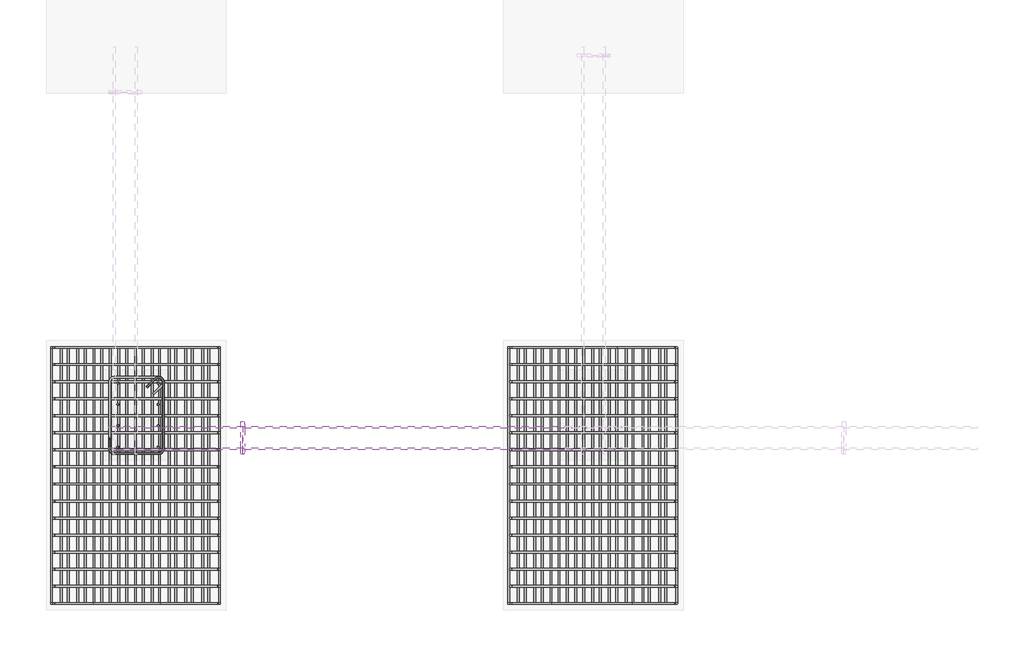
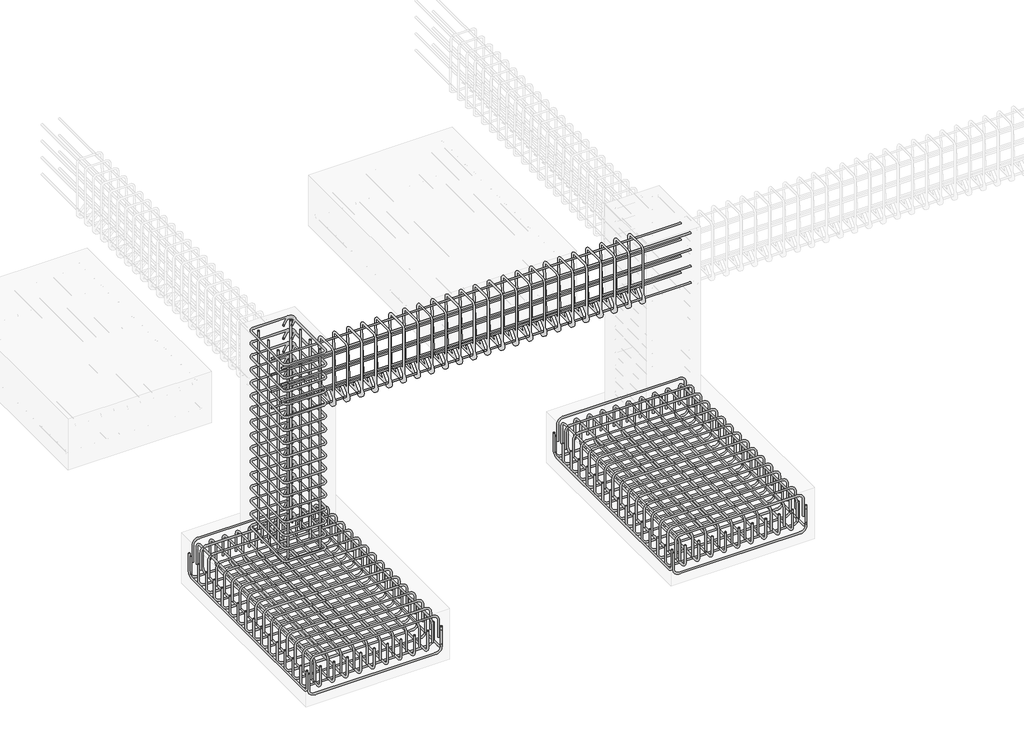
# One storey, part 2 of 16: 14 reinforcing bars.
"""IFC4 building model written with IfcOpenShell, lengths in millimetres."""

from ifc_helpers import new_model, si_unit, point, frame, origin, place, context, project, spatial, polyline, circle_curve, trimmed, segment, composite_curve, source, transform, mapped, element, save
from ifc_brep_helpers import swept_disk

model = new_model("IFC4")

# Units and contexts
model_context = context("Model", 3, world=origin())
ifc_project = project(units=[si_unit("LENGTHUNIT", "METRE", prefix="MILLI")], contexts=[model_context])

# Site, building, storey
site = spatial("IfcSite", under=ifc_project)
building = spatial("IfcBuilding", under=site)
storey = spatial("IfcBuildingStorey", under=building, Elevation=-1828.8)

# Reinforcing bars
placement = place(None, origin())
reinforcing_bar_shape = source(origin(), model_context, "Body", "SolidModel", [
    swept_disk(composite_curve([segment(polyline([(-4822.4802026, -711.9348046, -2028.4710597), (-4822.4802026, -711.9348046, -2175.7710597)]), True, "CONTINUOUS"), segment(trimmed(circle_curve(frame((-4868.8302026, -711.9348046, -2175.7710597), z_axis=(0.0, 1.0, 0.0), x_axis=(46.350000000000364, 0.0, 0.0)), 46.35), [point((-4822.4802026, -711.9348046, -2175.7710597))], [point((-4868.8302026, -711.9348046, -2222.1210597))], True, "CARTESIAN"), True, "CONTINUOUS"), segment(polyline([(-4868.8302026, -711.9348046, -2222.1210597), (-5883.4302026, -711.9348046, -2222.1210597)]), True, "CONTINUOUS"), segment(trimmed(circle_curve(frame((-5883.4302026, -711.9348046, -2175.7710597), z_axis=(0.0, 1.0, 0.0), x_axis=(0.0, 0.0, -46.34999999999991)), 46.35), [point((-5883.4302026, -711.9348046, -2222.1210597))], [point((-5929.7802026, -711.9348046, -2175.7710597))], True, "CARTESIAN"), True, "CONTINUOUS"), segment(polyline([(-5929.7802026, -711.9348046, -2175.7710597), (-5929.7802026, -711.9348046, -2028.4710597)]), True, "CONTINUOUS")], self_intersect=False), 6.35),
])
element("IfcReinforcingBar", 1, at=placement, inside=storey, context=model_context, shape_type="MappedRepresentation", body=[
    mapped(reinforcing_bar_shape, transform((0.0, 0.0, 0.0), x_axis=(1.0, 0.0, 0.0), y_axis=(0.0, 1.0, 0.0), z_axis=(0.0, 0.0, 1.0))),
    mapped(reinforcing_bar_shape, transform((0.0, -113.82, 0.0), x_axis=(1.0, 0.0, 0.0), y_axis=(0.0, 1.0, 0.0), z_axis=(0.0, 0.0, 1.0))),
    mapped(reinforcing_bar_shape, transform((0.0, -227.64, 0.0), x_axis=(1.0, 0.0, 0.0), y_axis=(0.0, 1.0, 0.0), z_axis=(0.0, 0.0, 1.0))),
    mapped(reinforcing_bar_shape, transform((0.0, -341.46, 0.0), x_axis=(1.0, 0.0, 0.0), y_axis=(0.0, 1.0, 0.0), z_axis=(0.0, 0.0, 1.0))),
    mapped(reinforcing_bar_shape, transform((0.0, -455.28, 0.0), x_axis=(1.0, 0.0, 0.0), y_axis=(0.0, 1.0, 0.0), z_axis=(0.0, 0.0, 1.0))),
    mapped(reinforcing_bar_shape, transform((0.0, -569.1, 0.0), x_axis=(1.0, 0.0, 0.0), y_axis=(0.0, 1.0, 0.0), z_axis=(0.0, 0.0, 1.0))),
    mapped(reinforcing_bar_shape, transform((0.0, -682.92, 0.0), x_axis=(1.0, 0.0, 0.0), y_axis=(0.0, 1.0, 0.0), z_axis=(0.0, 0.0, 1.0))),
    mapped(reinforcing_bar_shape, transform((0.0, -796.74, 0.0), x_axis=(1.0, 0.0, 0.0), y_axis=(0.0, 1.0, 0.0), z_axis=(0.0, 0.0, 1.0))),
    mapped(reinforcing_bar_shape, transform((0.0, -910.56, 0.0), x_axis=(1.0, 0.0, 0.0), y_axis=(0.0, 1.0, 0.0), z_axis=(0.0, 0.0, 1.0))),
    mapped(reinforcing_bar_shape, transform((0.0, -1024.38, 0.0), x_axis=(1.0, 0.0, 0.0), y_axis=(0.0, 1.0, 0.0), z_axis=(0.0, 0.0, 1.0))),
    mapped(reinforcing_bar_shape, transform((0.0, -1138.2, 0.0), x_axis=(1.0, 0.0, 0.0), y_axis=(0.0, 1.0, 0.0), z_axis=(0.0, 0.0, 1.0))),
    mapped(reinforcing_bar_shape, transform((0.0, -1252.02, 0.0), x_axis=(1.0, 0.0, 0.0), y_axis=(0.0, 1.0, 0.0), z_axis=(0.0, 0.0, 1.0))),
    mapped(reinforcing_bar_shape, transform((0.0, -1365.84, 0.0), x_axis=(1.0, 0.0, 0.0), y_axis=(0.0, 1.0, 0.0), z_axis=(0.0, 0.0, 1.0))),
    mapped(reinforcing_bar_shape, transform((0.0, -1479.66, 0.0), x_axis=(1.0, 0.0, 0.0), y_axis=(0.0, 1.0, 0.0), z_axis=(0.0, 0.0, 1.0))),
    mapped(reinforcing_bar_shape, transform((0.0, -1593.48, 0.0), x_axis=(1.0, 0.0, 0.0), y_axis=(0.0, 1.0, 0.0), z_axis=(0.0, 0.0, 1.0))),
    mapped(reinforcing_bar_shape, transform((0.0, -1707.3, 0.0), x_axis=(1.0, 0.0, 0.0), y_axis=(0.0, 1.0, 0.0), z_axis=(0.0, 0.0, 1.0))),
])
reinforcing_bar_2_shape = source(origin(), model_context, "Body", "SolidModel", [
    swept_disk(composite_curve([segment(polyline([(-5911.3242766, -711.9348046, -2081.4939987), (-5911.3242766, -711.9348046, -1934.1939987)]), True, "CONTINUOUS"), segment(trimmed(circle_curve(frame((-5864.9742766, -711.9348046, -1934.1939987), z_axis=(0.0, 1.0, 0.0), x_axis=(-46.350000000000364, 0.0, 0.0)), 46.35), [point((-5911.3242766, -711.9348046, -1934.1939987))], [point((-5864.9742766, -711.9348046, -1887.8439987))], True, "CARTESIAN"), True, "CONTINUOUS"), segment(polyline([(-5864.9742766, -711.9348046, -1887.8439987), (-4891.2549298, -711.9348046, -1887.8439987)]), True, "CONTINUOUS"), segment(trimmed(circle_curve(frame((-4891.2549298, -711.9348046, -1934.1939987), z_axis=(0.0, 1.0, 0.0), x_axis=(0.0, 0.0, 46.350000000000136)), 46.35), [point((-4891.2549298, -711.9348046, -1887.8439987))], [point((-4844.9049298, -711.9348046, -1934.1939987))], True, "CARTESIAN"), True, "CONTINUOUS"), segment(polyline([(-4844.9049298, -711.9348046, -1934.1939987), (-4844.9049298, -711.9348046, -2081.4939987)]), True, "CONTINUOUS")], self_intersect=False), 6.35),
])
element("IfcReinforcingBar", 2, at=placement, inside=storey, context=model_context, shape_type="MappedRepresentation", body=[
    mapped(reinforcing_bar_2_shape, transform((0.0, 0.0, 0.0), x_axis=(1.0, 0.0, 0.0), y_axis=(0.0, 1.0, 0.0), z_axis=(0.0, 0.0, 1.0))),
    mapped(reinforcing_bar_2_shape, transform((0.0, -113.82, 0.0), x_axis=(1.0, 0.0, 0.0), y_axis=(0.0, 1.0, 0.0), z_axis=(0.0, 0.0, 1.0))),
    mapped(reinforcing_bar_2_shape, transform((0.0, -227.64, 0.0), x_axis=(1.0, 0.0, 0.0), y_axis=(0.0, 1.0, 0.0), z_axis=(0.0, 0.0, 1.0))),
    mapped(reinforcing_bar_2_shape, transform((0.0, -341.46, 0.0), x_axis=(1.0, 0.0, 0.0), y_axis=(0.0, 1.0, 0.0), z_axis=(0.0, 0.0, 1.0))),
    mapped(reinforcing_bar_2_shape, transform((0.0, -455.28, 0.0), x_axis=(1.0, 0.0, 0.0), y_axis=(0.0, 1.0, 0.0), z_axis=(0.0, 0.0, 1.0))),
    mapped(reinforcing_bar_2_shape, transform((0.0, -569.1, 0.0), x_axis=(1.0, 0.0, 0.0), y_axis=(0.0, 1.0, 0.0), z_axis=(0.0, 0.0, 1.0))),
    mapped(reinforcing_bar_2_shape, transform((0.0, -682.92, 0.0), x_axis=(1.0, 0.0, 0.0), y_axis=(0.0, 1.0, 0.0), z_axis=(0.0, 0.0, 1.0))),
    mapped(reinforcing_bar_2_shape, transform((0.0, -796.74, 0.0), x_axis=(1.0, 0.0, 0.0), y_axis=(0.0, 1.0, 0.0), z_axis=(0.0, 0.0, 1.0))),
    mapped(reinforcing_bar_2_shape, transform((0.0, -910.56, 0.0), x_axis=(1.0, 0.0, 0.0), y_axis=(0.0, 1.0, 0.0), z_axis=(0.0, 0.0, 1.0))),
    mapped(reinforcing_bar_2_shape, transform((0.0, -1024.38, 0.0), x_axis=(1.0, 0.0, 0.0), y_axis=(0.0, 1.0, 0.0), z_axis=(0.0, 0.0, 1.0))),
    mapped(reinforcing_bar_2_shape, transform((0.0, -1138.2, 0.0), x_axis=(1.0, 0.0, 0.0), y_axis=(0.0, 1.0, 0.0), z_axis=(0.0, 0.0, 1.0))),
    mapped(reinforcing_bar_2_shape, transform((0.0, -1252.02, 0.0), x_axis=(1.0, 0.0, 0.0), y_axis=(0.0, 1.0, 0.0), z_axis=(0.0, 0.0, 1.0))),
    mapped(reinforcing_bar_2_shape, transform((0.0, -1365.84, 0.0), x_axis=(1.0, 0.0, 0.0), y_axis=(0.0, 1.0, 0.0), z_axis=(0.0, 0.0, 1.0))),
    mapped(reinforcing_bar_2_shape, transform((0.0, -1479.66, 0.0), x_axis=(1.0, 0.0, 0.0), y_axis=(0.0, 1.0, 0.0), z_axis=(0.0, 0.0, 1.0))),
    mapped(reinforcing_bar_2_shape, transform((0.0, -1593.48, 0.0), x_axis=(1.0, 0.0, 0.0), y_axis=(0.0, 1.0, 0.0), z_axis=(0.0, 0.0, 1.0))),
    mapped(reinforcing_bar_2_shape, transform((0.0, -1707.3, 0.0), x_axis=(1.0, 0.0, 0.0), y_axis=(0.0, 1.0, 0.0), z_axis=(0.0, 0.0, 1.0))),
])
reinforcing_bar_3_shape = source(origin(), model_context, "Body", "SolidModel", [
    swept_disk(composite_curve([segment(polyline([(-4894.8565936, -711.9348046, -2112.6585679), (-4894.8565936, -711.9348046, -1965.3585679)]), True, "CONTINUOUS"), segment(trimmed(circle_curve(frame((-4894.8565936, -758.2848046, -1965.3585679), z_axis=(1.0, 0.0, 0.0), x_axis=(0.0, 46.35000000000002, 0.0)), 46.35), [point((-4894.8565936, -711.9348046, -1965.3585679))], [point((-4894.8565936, -758.2848046, -1919.0085679))], True, "CARTESIAN"), True, "CONTINUOUS"), segment(polyline([(-4894.8565936, -758.2848046, -1919.0085679), (-4894.8565936, -2372.8848046, -1919.0085679)]), True, "CONTINUOUS"), segment(trimmed(circle_curve(frame((-4894.8565936, -2372.8848046, -1965.3585679), z_axis=(1.0, 0.0, 0.0), x_axis=(0.0, 0.0, 46.350000000000136)), 46.35), [point((-4894.8565936, -2372.8848046, -1919.0085679))], [point((-4894.8565936, -2419.2348046, -1965.3585679))], True, "CARTESIAN"), True, "CONTINUOUS"), segment(polyline([(-4894.8565936, -2419.2348046, -1965.3585679), (-4894.8565936, -2419.2348046, -2112.6585679)]), True, "CONTINUOUS")], self_intersect=False), 6.35),
])
element("IfcReinforcingBar", 3, at=placement, inside=storey, context=model_context, shape_type="MappedRepresentation", body=[
    mapped(reinforcing_bar_3_shape, transform((0.0, 0.0, 0.0), x_axis=(1.0, 0.0, 0.0), y_axis=(0.0, 1.0, 0.0), z_axis=(0.0, 0.0, 1.0))),
    mapped(reinforcing_bar_3_shape, transform((-109.2679104, 0.0, 0.0), x_axis=(1.0, 0.0, 0.0), y_axis=(0.0, 1.0, 0.0), z_axis=(0.0, 0.0, 1.0))),
    mapped(reinforcing_bar_3_shape, transform((-218.5358207, 0.0, 0.0), x_axis=(1.0, 0.0, 0.0), y_axis=(0.0, 1.0, 0.0), z_axis=(0.0, 0.0, 1.0))),
    mapped(reinforcing_bar_3_shape, transform((-327.8037311, 0.0, 0.0), x_axis=(1.0, 0.0, 0.0), y_axis=(0.0, 1.0, 0.0), z_axis=(0.0, 0.0, 1.0))),
    mapped(reinforcing_bar_3_shape, transform((-437.0716415, 0.0, 0.0), x_axis=(1.0, 0.0, 0.0), y_axis=(0.0, 1.0, 0.0), z_axis=(0.0, 0.0, 1.0))),
    mapped(reinforcing_bar_3_shape, transform((-546.3395518, 0.0, 0.0), x_axis=(1.0, 0.0, 0.0), y_axis=(0.0, 1.0, 0.0), z_axis=(0.0, 0.0, 1.0))),
    mapped(reinforcing_bar_3_shape, transform((-655.6074622, 0.0, 0.0), x_axis=(1.0, 0.0, 0.0), y_axis=(0.0, 1.0, 0.0), z_axis=(0.0, 0.0, 1.0))),
    mapped(reinforcing_bar_3_shape, transform((-764.8753726, 0.0, 0.0), x_axis=(1.0, 0.0, 0.0), y_axis=(0.0, 1.0, 0.0), z_axis=(0.0, 0.0, 1.0))),
    mapped(reinforcing_bar_3_shape, transform((-874.1432829, 0.0, 0.0), x_axis=(1.0, 0.0, 0.0), y_axis=(0.0, 1.0, 0.0), z_axis=(0.0, 0.0, 1.0))),
    mapped(reinforcing_bar_3_shape, transform((-983.4111933, 0.0, 0.0), x_axis=(1.0, 0.0, 0.0), y_axis=(0.0, 1.0, 0.0), z_axis=(0.0, 0.0, 1.0))),
])
reinforcing_bar_4_shape = source(origin(), model_context, "Body", "SolidModel", [
    swept_disk(composite_curve([segment(polyline([(-5943.0342668, -711.9348046, -1996.4434391), (-5943.0342668, -711.9348046, -2143.7434391)]), True, "CONTINUOUS"), segment(trimmed(circle_curve(frame((-5943.0342668, -758.2848046, -2143.7434391), z_axis=(-1.0, 0.0, 0.0), x_axis=(0.0, 46.35000000000002, 0.0)), 46.35), [point((-5943.0342668, -711.9348046, -2143.7434391))], [point((-5943.0342668, -758.2848046, -2190.0934391))], True, "CARTESIAN"), True, "CONTINUOUS"), segment(polyline([(-5943.0342668, -758.2848046, -2190.0934391), (-5943.0342668, -2372.8848046, -2190.0934391)]), True, "CONTINUOUS"), segment(trimmed(circle_curve(frame((-5943.0342668, -2372.8848046, -2143.7434391), z_axis=(-1.0, 0.0, 0.0), x_axis=(0.0, 0.0, -46.34999999999991)), 46.35), [point((-5943.0342668, -2372.8848046, -2190.0934391))], [point((-5943.0342668, -2419.2348046, -2143.7434391))], True, "CARTESIAN"), True, "CONTINUOUS"), segment(polyline([(-5943.0342668, -2419.2348046, -2143.7434391), (-5943.0342668, -2419.2348046, -1996.4434391)]), True, "CONTINUOUS")], self_intersect=False), 6.35),
])
element("IfcReinforcingBar", 4, at=placement, inside=storey, context=model_context, shape_type="MappedRepresentation", body=[
    mapped(reinforcing_bar_4_shape, transform((0.0, 0.0, 0.0), x_axis=(1.0, 0.0, 0.0), y_axis=(0.0, 1.0, 0.0), z_axis=(0.0, 0.0, 1.0))),
    mapped(reinforcing_bar_4_shape, transform((112.0554064, 0.0, 0.0), x_axis=(1.0, 0.0, 0.0), y_axis=(0.0, 1.0, 0.0), z_axis=(0.0, 0.0, 1.0))),
    mapped(reinforcing_bar_4_shape, transform((224.1108128, 0.0, 0.0), x_axis=(1.0, 0.0, 0.0), y_axis=(0.0, 1.0, 0.0), z_axis=(0.0, 0.0, 1.0))),
    mapped(reinforcing_bar_4_shape, transform((336.1662192, 0.0, 0.0), x_axis=(1.0, 0.0, 0.0), y_axis=(0.0, 1.0, 0.0), z_axis=(0.0, 0.0, 1.0))),
    mapped(reinforcing_bar_4_shape, transform((448.2216256, 0.0, 0.0), x_axis=(1.0, 0.0, 0.0), y_axis=(0.0, 1.0, 0.0), z_axis=(0.0, 0.0, 1.0))),
    mapped(reinforcing_bar_4_shape, transform((560.2770321, 0.0, 0.0), x_axis=(1.0, 0.0, 0.0), y_axis=(0.0, 1.0, 0.0), z_axis=(0.0, 0.0, 1.0))),
    mapped(reinforcing_bar_4_shape, transform((672.3324385, 0.0, 0.0), x_axis=(1.0, 0.0, 0.0), y_axis=(0.0, 1.0, 0.0), z_axis=(0.0, 0.0, 1.0))),
    mapped(reinforcing_bar_4_shape, transform((784.3878449, 0.0, 0.0), x_axis=(1.0, 0.0, 0.0), y_axis=(0.0, 1.0, 0.0), z_axis=(0.0, 0.0, 1.0))),
    mapped(reinforcing_bar_4_shape, transform((896.4432513, 0.0, 0.0), x_axis=(1.0, 0.0, 0.0), y_axis=(0.0, 1.0, 0.0), z_axis=(0.0, 0.0, 1.0))),
    mapped(reinforcing_bar_4_shape, transform((1008.4986577, 0.0, 0.0), x_axis=(1.0, 0.0, 0.0), y_axis=(0.0, 1.0, 0.0), z_axis=(0.0, 0.0, 1.0))),
    mapped(reinforcing_bar_4_shape, transform((1120.5540641, 0.0, 0.0), x_axis=(1.0, 0.0, 0.0), y_axis=(0.0, 1.0, 0.0), z_axis=(0.0, 0.0, 1.0))),
])
reinforcing_bar_5_shape = source(origin(), model_context, "Body", "SolidModel", [
    swept_disk(composite_curve([segment(polyline([(-1774.4802026, -711.9348046, -2028.4710597), (-1774.4802026, -711.9348046, -2175.7710597)]), True, "CONTINUOUS"), segment(trimmed(circle_curve(frame((-1820.8302026, -711.9348046, -2175.7710597), z_axis=(0.0, 1.0, 0.0), x_axis=(46.34999999999991, 0.0, 0.0)), 46.35), [point((-1774.4802026, -711.9348046, -2175.7710597))], [point((-1820.8302026, -711.9348046, -2222.1210597))], True, "CARTESIAN"), True, "CONTINUOUS"), segment(polyline([(-1820.8302026, -711.9348046, -2222.1210597), (-2835.4302026, -711.9348046, -2222.1210597)]), True, "CONTINUOUS"), segment(trimmed(circle_curve(frame((-2835.4302026, -711.9348046, -2175.7710597), z_axis=(0.0, 1.0, 0.0), x_axis=(0.0, 0.0, -46.34999999999991)), 46.35), [point((-2835.4302026, -711.9348046, -2222.1210597))], [point((-2881.7802026, -711.9348046, -2175.7710597))], True, "CARTESIAN"), True, "CONTINUOUS"), segment(polyline([(-2881.7802026, -711.9348046, -2175.7710597), (-2881.7802026, -711.9348046, -2028.4710597)]), True, "CONTINUOUS")], self_intersect=False), 6.35),
])
element("IfcReinforcingBar", 5, at=placement, inside=storey, context=model_context, shape_type="MappedRepresentation", body=[
    mapped(reinforcing_bar_5_shape, transform((0.0, 0.0, 0.0), x_axis=(1.0, 0.0, 0.0), y_axis=(0.0, 1.0, 0.0), z_axis=(0.0, 0.0, 1.0))),
    mapped(reinforcing_bar_5_shape, transform((0.0, -113.82, 0.0), x_axis=(1.0, 0.0, 0.0), y_axis=(0.0, 1.0, 0.0), z_axis=(0.0, 0.0, 1.0))),
    mapped(reinforcing_bar_5_shape, transform((0.0, -227.64, 0.0), x_axis=(1.0, 0.0, 0.0), y_axis=(0.0, 1.0, 0.0), z_axis=(0.0, 0.0, 1.0))),
    mapped(reinforcing_bar_5_shape, transform((0.0, -341.46, 0.0), x_axis=(1.0, 0.0, 0.0), y_axis=(0.0, 1.0, 0.0), z_axis=(0.0, 0.0, 1.0))),
    mapped(reinforcing_bar_5_shape, transform((0.0, -455.28, 0.0), x_axis=(1.0, 0.0, 0.0), y_axis=(0.0, 1.0, 0.0), z_axis=(0.0, 0.0, 1.0))),
    mapped(reinforcing_bar_5_shape, transform((0.0, -569.1, 0.0), x_axis=(1.0, 0.0, 0.0), y_axis=(0.0, 1.0, 0.0), z_axis=(0.0, 0.0, 1.0))),
    mapped(reinforcing_bar_5_shape, transform((0.0, -682.92, 0.0), x_axis=(1.0, 0.0, 0.0), y_axis=(0.0, 1.0, 0.0), z_axis=(0.0, 0.0, 1.0))),
    mapped(reinforcing_bar_5_shape, transform((0.0, -796.74, 0.0), x_axis=(1.0, 0.0, 0.0), y_axis=(0.0, 1.0, 0.0), z_axis=(0.0, 0.0, 1.0))),
    mapped(reinforcing_bar_5_shape, transform((0.0, -910.56, 0.0), x_axis=(1.0, 0.0, 0.0), y_axis=(0.0, 1.0, 0.0), z_axis=(0.0, 0.0, 1.0))),
    mapped(reinforcing_bar_5_shape, transform((0.0, -1024.38, 0.0), x_axis=(1.0, 0.0, 0.0), y_axis=(0.0, 1.0, 0.0), z_axis=(0.0, 0.0, 1.0))),
    mapped(reinforcing_bar_5_shape, transform((0.0, -1138.2, 0.0), x_axis=(1.0, 0.0, 0.0), y_axis=(0.0, 1.0, 0.0), z_axis=(0.0, 0.0, 1.0))),
    mapped(reinforcing_bar_5_shape, transform((0.0, -1252.02, 0.0), x_axis=(1.0, 0.0, 0.0), y_axis=(0.0, 1.0, 0.0), z_axis=(0.0, 0.0, 1.0))),
    mapped(reinforcing_bar_5_shape, transform((0.0, -1365.84, 0.0), x_axis=(1.0, 0.0, 0.0), y_axis=(0.0, 1.0, 0.0), z_axis=(0.0, 0.0, 1.0))),
    mapped(reinforcing_bar_5_shape, transform((0.0, -1479.66, 0.0), x_axis=(1.0, 0.0, 0.0), y_axis=(0.0, 1.0, 0.0), z_axis=(0.0, 0.0, 1.0))),
    mapped(reinforcing_bar_5_shape, transform((0.0, -1593.48, 0.0), x_axis=(1.0, 0.0, 0.0), y_axis=(0.0, 1.0, 0.0), z_axis=(0.0, 0.0, 1.0))),
    mapped(reinforcing_bar_5_shape, transform((0.0, -1707.3, 0.0), x_axis=(1.0, 0.0, 0.0), y_axis=(0.0, 1.0, 0.0), z_axis=(0.0, 0.0, 1.0))),
])
reinforcing_bar_6_shape = source(origin(), model_context, "Body", "SolidModel", [
    swept_disk(composite_curve([segment(polyline([(-2863.3242766, -711.9348046, -2081.4939987), (-2863.3242766, -711.9348046, -1934.1939987)]), True, "CONTINUOUS"), segment(trimmed(circle_curve(frame((-2816.9742766, -711.9348046, -1934.1939987), z_axis=(0.0, 1.0, 0.0), x_axis=(-46.34999999999991, 0.0, 0.0)), 46.35), [point((-2863.3242766, -711.9348046, -1934.1939987))], [point((-2816.9742766, -711.9348046, -1887.8439987))], True, "CARTESIAN"), True, "CONTINUOUS"), segment(polyline([(-2816.9742766, -711.9348046, -1887.8439987), (-1843.2549298, -711.9348046, -1887.8439987)]), True, "CONTINUOUS"), segment(trimmed(circle_curve(frame((-1843.2549298, -711.9348046, -1934.1939987), z_axis=(0.0, 1.0, 0.0), x_axis=(0.0, 0.0, 46.350000000000136)), 46.35), [point((-1843.2549298, -711.9348046, -1887.8439987))], [point((-1796.9049298, -711.9348046, -1934.1939987))], True, "CARTESIAN"), True, "CONTINUOUS"), segment(polyline([(-1796.9049298, -711.9348046, -1934.1939987), (-1796.9049298, -711.9348046, -2081.4939987)]), True, "CONTINUOUS")], self_intersect=False), 6.35),
])
element("IfcReinforcingBar", 6, at=placement, inside=storey, context=model_context, shape_type="MappedRepresentation", body=[
    mapped(reinforcing_bar_6_shape, transform((0.0, 0.0, 0.0), x_axis=(1.0, 0.0, 0.0), y_axis=(0.0, 1.0, 0.0), z_axis=(0.0, 0.0, 1.0))),
    mapped(reinforcing_bar_6_shape, transform((0.0, -113.82, 0.0), x_axis=(1.0, 0.0, 0.0), y_axis=(0.0, 1.0, 0.0), z_axis=(0.0, 0.0, 1.0))),
    mapped(reinforcing_bar_6_shape, transform((0.0, -227.64, 0.0), x_axis=(1.0, 0.0, 0.0), y_axis=(0.0, 1.0, 0.0), z_axis=(0.0, 0.0, 1.0))),
    mapped(reinforcing_bar_6_shape, transform((0.0, -341.46, 0.0), x_axis=(1.0, 0.0, 0.0), y_axis=(0.0, 1.0, 0.0), z_axis=(0.0, 0.0, 1.0))),
    mapped(reinforcing_bar_6_shape, transform((0.0, -455.28, 0.0), x_axis=(1.0, 0.0, 0.0), y_axis=(0.0, 1.0, 0.0), z_axis=(0.0, 0.0, 1.0))),
    mapped(reinforcing_bar_6_shape, transform((0.0, -569.1, 0.0), x_axis=(1.0, 0.0, 0.0), y_axis=(0.0, 1.0, 0.0), z_axis=(0.0, 0.0, 1.0))),
    mapped(reinforcing_bar_6_shape, transform((0.0, -682.92, 0.0), x_axis=(1.0, 0.0, 0.0), y_axis=(0.0, 1.0, 0.0), z_axis=(0.0, 0.0, 1.0))),
    mapped(reinforcing_bar_6_shape, transform((0.0, -796.74, 0.0), x_axis=(1.0, 0.0, 0.0), y_axis=(0.0, 1.0, 0.0), z_axis=(0.0, 0.0, 1.0))),
    mapped(reinforcing_bar_6_shape, transform((0.0, -910.56, 0.0), x_axis=(1.0, 0.0, 0.0), y_axis=(0.0, 1.0, 0.0), z_axis=(0.0, 0.0, 1.0))),
    mapped(reinforcing_bar_6_shape, transform((0.0, -1024.38, 0.0), x_axis=(1.0, 0.0, 0.0), y_axis=(0.0, 1.0, 0.0), z_axis=(0.0, 0.0, 1.0))),
    mapped(reinforcing_bar_6_shape, transform((0.0, -1138.2, 0.0), x_axis=(1.0, 0.0, 0.0), y_axis=(0.0, 1.0, 0.0), z_axis=(0.0, 0.0, 1.0))),
    mapped(reinforcing_bar_6_shape, transform((0.0, -1252.02, 0.0), x_axis=(1.0, 0.0, 0.0), y_axis=(0.0, 1.0, 0.0), z_axis=(0.0, 0.0, 1.0))),
    mapped(reinforcing_bar_6_shape, transform((0.0, -1365.84, 0.0), x_axis=(1.0, 0.0, 0.0), y_axis=(0.0, 1.0, 0.0), z_axis=(0.0, 0.0, 1.0))),
    mapped(reinforcing_bar_6_shape, transform((0.0, -1479.66, 0.0), x_axis=(1.0, 0.0, 0.0), y_axis=(0.0, 1.0, 0.0), z_axis=(0.0, 0.0, 1.0))),
    mapped(reinforcing_bar_6_shape, transform((0.0, -1593.48, 0.0), x_axis=(1.0, 0.0, 0.0), y_axis=(0.0, 1.0, 0.0), z_axis=(0.0, 0.0, 1.0))),
    mapped(reinforcing_bar_6_shape, transform((0.0, -1707.3, 0.0), x_axis=(1.0, 0.0, 0.0), y_axis=(0.0, 1.0, 0.0), z_axis=(0.0, 0.0, 1.0))),
])
reinforcing_bar_7_shape = source(origin(), model_context, "Body", "SolidModel", [
    swept_disk(composite_curve([segment(polyline([(-1846.8565936, -711.9348046, -2112.6585679), (-1846.8565936, -711.9348046, -1965.3585679)]), True, "CONTINUOUS"), segment(trimmed(circle_curve(frame((-1846.8565936, -758.2848046, -1965.3585679), z_axis=(1.0, 0.0, 0.0), x_axis=(0.0, 46.35000000000002, 0.0)), 46.35), [point((-1846.8565936, -711.9348046, -1965.3585679))], [point((-1846.8565936, -758.2848046, -1919.0085679))], True, "CARTESIAN"), True, "CONTINUOUS"), segment(polyline([(-1846.8565936, -758.2848046, -1919.0085679), (-1846.8565936, -2372.8848046, -1919.0085679)]), True, "CONTINUOUS"), segment(trimmed(circle_curve(frame((-1846.8565936, -2372.8848046, -1965.3585679), z_axis=(1.0, 0.0, 0.0), x_axis=(0.0, 0.0, 46.350000000000136)), 46.35), [point((-1846.8565936, -2372.8848046, -1919.0085679))], [point((-1846.8565936, -2419.2348046, -1965.3585679))], True, "CARTESIAN"), True, "CONTINUOUS"), segment(polyline([(-1846.8565936, -2419.2348046, -1965.3585679), (-1846.8565936, -2419.2348046, -2112.6585679)]), True, "CONTINUOUS")], self_intersect=False), 6.35),
])
element("IfcReinforcingBar", 7, at=placement, inside=storey, context=model_context, shape_type="MappedRepresentation", body=[
    mapped(reinforcing_bar_7_shape, transform((0.0, 0.0, 0.0), x_axis=(1.0, 0.0, 0.0), y_axis=(0.0, 1.0, 0.0), z_axis=(0.0, 0.0, 1.0))),
    mapped(reinforcing_bar_7_shape, transform((-109.2679104, 0.0, 0.0), x_axis=(1.0, 0.0, 0.0), y_axis=(0.0, 1.0, 0.0), z_axis=(0.0, 0.0, 1.0))),
    mapped(reinforcing_bar_7_shape, transform((-218.5358207, 0.0, 0.0), x_axis=(1.0, 0.0, 0.0), y_axis=(0.0, 1.0, 0.0), z_axis=(0.0, 0.0, 1.0))),
    mapped(reinforcing_bar_7_shape, transform((-327.8037311, 0.0, 0.0), x_axis=(1.0, 0.0, 0.0), y_axis=(0.0, 1.0, 0.0), z_axis=(0.0, 0.0, 1.0))),
    mapped(reinforcing_bar_7_shape, transform((-437.0716415, 0.0, 0.0), x_axis=(1.0, 0.0, 0.0), y_axis=(0.0, 1.0, 0.0), z_axis=(0.0, 0.0, 1.0))),
    mapped(reinforcing_bar_7_shape, transform((-546.3395518, 0.0, 0.0), x_axis=(1.0, 0.0, 0.0), y_axis=(0.0, 1.0, 0.0), z_axis=(0.0, 0.0, 1.0))),
    mapped(reinforcing_bar_7_shape, transform((-655.6074622, 0.0, 0.0), x_axis=(1.0, 0.0, 0.0), y_axis=(0.0, 1.0, 0.0), z_axis=(0.0, 0.0, 1.0))),
    mapped(reinforcing_bar_7_shape, transform((-764.8753726, 0.0, 0.0), x_axis=(1.0, 0.0, 0.0), y_axis=(0.0, 1.0, 0.0), z_axis=(0.0, 0.0, 1.0))),
    mapped(reinforcing_bar_7_shape, transform((-874.1432829, 0.0, 0.0), x_axis=(1.0, 0.0, 0.0), y_axis=(0.0, 1.0, 0.0), z_axis=(0.0, 0.0, 1.0))),
    mapped(reinforcing_bar_7_shape, transform((-983.4111933, 0.0, 0.0), x_axis=(1.0, 0.0, 0.0), y_axis=(0.0, 1.0, 0.0), z_axis=(0.0, 0.0, 1.0))),
])
reinforcing_bar_8_shape = source(origin(), model_context, "Body", "SolidModel", [
    swept_disk(composite_curve([segment(polyline([(-2895.0342668, -711.9348046, -1996.4434391), (-2895.0342668, -711.9348046, -2143.7434391)]), True, "CONTINUOUS"), segment(trimmed(circle_curve(frame((-2895.0342668, -758.2848046, -2143.7434391), z_axis=(-1.0, 0.0, 0.0), x_axis=(0.0, 46.35000000000002, 0.0)), 46.35), [point((-2895.0342668, -711.9348046, -2143.7434391))], [point((-2895.0342668, -758.2848046, -2190.0934391))], True, "CARTESIAN"), True, "CONTINUOUS"), segment(polyline([(-2895.0342668, -758.2848046, -2190.0934391), (-2895.0342668, -2372.8848046, -2190.0934391)]), True, "CONTINUOUS"), segment(trimmed(circle_curve(frame((-2895.0342668, -2372.8848046, -2143.7434391), z_axis=(-1.0, 0.0, 0.0), x_axis=(0.0, 0.0, -46.34999999999991)), 46.35), [point((-2895.0342668, -2372.8848046, -2190.0934391))], [point((-2895.0342668, -2419.2348046, -2143.7434391))], True, "CARTESIAN"), True, "CONTINUOUS"), segment(polyline([(-2895.0342668, -2419.2348046, -2143.7434391), (-2895.0342668, -2419.2348046, -1996.4434391)]), True, "CONTINUOUS")], self_intersect=False), 6.35),
])
element("IfcReinforcingBar", 8, at=placement, inside=storey, context=model_context, shape_type="MappedRepresentation", body=[
    mapped(reinforcing_bar_8_shape, transform((0.0, 0.0, 0.0), x_axis=(1.0, 0.0, 0.0), y_axis=(0.0, 1.0, 0.0), z_axis=(0.0, 0.0, 1.0))),
    mapped(reinforcing_bar_8_shape, transform((112.0554064, 0.0, 0.0), x_axis=(1.0, 0.0, 0.0), y_axis=(0.0, 1.0, 0.0), z_axis=(0.0, 0.0, 1.0))),
    mapped(reinforcing_bar_8_shape, transform((224.1108128, 0.0, 0.0), x_axis=(1.0, 0.0, 0.0), y_axis=(0.0, 1.0, 0.0), z_axis=(0.0, 0.0, 1.0))),
    mapped(reinforcing_bar_8_shape, transform((336.1662192, 0.0, 0.0), x_axis=(1.0, 0.0, 0.0), y_axis=(0.0, 1.0, 0.0), z_axis=(0.0, 0.0, 1.0))),
    mapped(reinforcing_bar_8_shape, transform((448.2216256, 0.0, 0.0), x_axis=(1.0, 0.0, 0.0), y_axis=(0.0, 1.0, 0.0), z_axis=(0.0, 0.0, 1.0))),
    mapped(reinforcing_bar_8_shape, transform((560.2770321, 0.0, 0.0), x_axis=(1.0, 0.0, 0.0), y_axis=(0.0, 1.0, 0.0), z_axis=(0.0, 0.0, 1.0))),
    mapped(reinforcing_bar_8_shape, transform((672.3324385, 0.0, 0.0), x_axis=(1.0, 0.0, 0.0), y_axis=(0.0, 1.0, 0.0), z_axis=(0.0, 0.0, 1.0))),
    mapped(reinforcing_bar_8_shape, transform((784.3878449, 0.0, 0.0), x_axis=(1.0, 0.0, 0.0), y_axis=(0.0, 1.0, 0.0), z_axis=(0.0, 0.0, 1.0))),
    mapped(reinforcing_bar_8_shape, transform((896.4432513, 0.0, 0.0), x_axis=(1.0, 0.0, 0.0), y_axis=(0.0, 1.0, 0.0), z_axis=(0.0, 0.0, 1.0))),
    mapped(reinforcing_bar_8_shape, transform((1008.4986577, 0.0, 0.0), x_axis=(1.0, 0.0, 0.0), y_axis=(0.0, 1.0, 0.0), z_axis=(0.0, 0.0, 1.0))),
    mapped(reinforcing_bar_8_shape, transform((1120.5540641, 0.0, 0.0), x_axis=(1.0, 0.0, 0.0), y_axis=(0.0, 1.0, 0.0), z_axis=(0.0, 0.0, 1.0))),
])
reinforcing_bar_9_shape = source(origin(), model_context, "Body", "SolidModel", [
    swept_disk(composite_curve([segment(polyline([(-5306.7415632, -976.86057, -46.35), (-5250.9980002, -921.117007, -46.35)]), True, "CONTINUOUS"), segment(trimmed(circle_curve(frame((-5228.8302026, -943.2848046, -46.35), z_axis=(0.0, 0.0, -1.0), x_axis=(-22.167797600000085, 22.167797600000085, 0.0)), 31.35), [point((-5250.9980002, -921.117007, -46.35))], [point((-5197.4802026, -943.2848046, -46.35))], True, "CARTESIAN"), True, "CONTINUOUS"), segment(polyline([(-5197.4802026, -943.2848046, -46.35), (-5197.4802026, -1387.8848046, -46.35)]), True, "CONTINUOUS"), segment(trimmed(circle_curve(frame((-5228.8302026, -1387.8848046, -46.35), z_axis=(0.0, 0.0, -1.0), x_axis=(31.350000000000364, 0.0, 0.0)), 31.35), [point((-5197.4802026, -1387.8848046, -46.35))], [point((-5228.8302026, -1419.2348046, -46.35))], True, "CARTESIAN"), True, "CONTINUOUS"), segment(polyline([(-5228.8302026, -1419.2348046, -46.35), (-5523.4302026, -1419.2348046, -46.35)]), True, "CONTINUOUS"), segment(trimmed(circle_curve(frame((-5523.4302026, -1387.8946239, -45.5654144), z_axis=(0.0, 0.025026655153786343, -0.9996867842138424), x_axis=(0.0, -31.34018070000002, -0.7845855999999998)), 31.35), [point((-5523.4302026, -1419.2348046, -46.35))], [point((-5554.7802026, -1387.8946239, -45.5654144))], True, "CARTESIAN"), True, "CONTINUOUS"), segment(polyline([(-5554.7802026, -1387.8946239, -45.5654144), (-5554.7802026, -943.2749853, -34.4345856)]), True, "CONTINUOUS"), segment(trimmed(circle_curve(frame((-5523.4302026, -943.2749853, -34.4345856), z_axis=(0.0, 0.025026655153786343, -0.9996867842138424), x_axis=(-31.350000000000364, 0.0, 0.0)), 31.35), [point((-5554.7802026, -943.2749853, -34.4345856))], [point((-5523.4302026, -911.9348046, -33.65))], True, "CARTESIAN"), True, "CONTINUOUS"), segment(polyline([(-5523.4302026, -911.9348046, -33.65), (-5228.8302026, -911.9348046, -33.65)]), True, "CONTINUOUS"), segment(trimmed(circle_curve(frame((-5228.8302026, -943.2848046, -33.65), z_axis=(0.0, 0.0, -1.0), x_axis=(0.0, 31.350000000000023, 0.0)), 31.35), [point((-5228.8302026, -911.9348046, -33.65))], [point((-5206.662405, -965.4526022, -33.65))], True, "CARTESIAN"), True, "CONTINUOUS"), segment(polyline([(-5206.662405, -965.4526022, -33.65), (-5262.405968, -1021.1961652, -33.65)]), True, "CONTINUOUS")], self_intersect=False), 6.35),
])
element("IfcReinforcingBar", 9, at=placement, inside=storey, context=model_context, shape_type="MappedRepresentation", body=[
    mapped(reinforcing_bar_9_shape, transform((0.0, 0.0, 0.0), x_axis=(1.0, 0.0, 0.0), y_axis=(0.0, 1.0, 0.0), z_axis=(0.0, 0.0, 1.0))),
    mapped(reinforcing_bar_9_shape, transform((0.0, 0.0, -115.74), x_axis=(1.0, 0.0, 0.0), y_axis=(0.0, 1.0, 0.0), z_axis=(0.0, 0.0, 1.0))),
    mapped(reinforcing_bar_9_shape, transform((0.0, 0.0, -231.48), x_axis=(1.0, 0.0, 0.0), y_axis=(0.0, 1.0, 0.0), z_axis=(0.0, 0.0, 1.0))),
    mapped(reinforcing_bar_9_shape, transform((0.0, 0.0, -347.22), x_axis=(1.0, 0.0, 0.0), y_axis=(0.0, 1.0, 0.0), z_axis=(0.0, 0.0, 1.0))),
    mapped(reinforcing_bar_9_shape, transform((0.0, 0.0, -462.96), x_axis=(1.0, 0.0, 0.0), y_axis=(0.0, 1.0, 0.0), z_axis=(0.0, 0.0, 1.0))),
    mapped(reinforcing_bar_9_shape, transform((0.0, 0.0, -578.7), x_axis=(1.0, 0.0, 0.0), y_axis=(0.0, 1.0, 0.0), z_axis=(0.0, 0.0, 1.0))),
    mapped(reinforcing_bar_9_shape, transform((0.0, 0.0, -694.44), x_axis=(1.0, 0.0, 0.0), y_axis=(0.0, 1.0, 0.0), z_axis=(0.0, 0.0, 1.0))),
    mapped(reinforcing_bar_9_shape, transform((0.0, 0.0, -810.18), x_axis=(1.0, 0.0, 0.0), y_axis=(0.0, 1.0, 0.0), z_axis=(0.0, 0.0, 1.0))),
    mapped(reinforcing_bar_9_shape, transform((0.0, 0.0, -925.92), x_axis=(1.0, 0.0, 0.0), y_axis=(0.0, 1.0, 0.0), z_axis=(0.0, 0.0, 1.0))),
    mapped(reinforcing_bar_9_shape, transform((0.0, 0.0, -1041.66), x_axis=(1.0, 0.0, 0.0), y_axis=(0.0, 1.0, 0.0), z_axis=(0.0, 0.0, 1.0))),
    mapped(reinforcing_bar_9_shape, transform((0.0, 0.0, -1157.4), x_axis=(1.0, 0.0, 0.0), y_axis=(0.0, 1.0, 0.0), z_axis=(0.0, 0.0, 1.0))),
    mapped(reinforcing_bar_9_shape, transform((0.0, 0.0, -1273.14), x_axis=(1.0, 0.0, 0.0), y_axis=(0.0, 1.0, 0.0), z_axis=(0.0, 0.0, 1.0))),
    mapped(reinforcing_bar_9_shape, transform((0.0, 0.0, -1388.88), x_axis=(1.0, 0.0, 0.0), y_axis=(0.0, 1.0, 0.0), z_axis=(0.0, 0.0, 1.0))),
    mapped(reinforcing_bar_9_shape, transform((0.0, 0.0, -1504.62), x_axis=(1.0, 0.0, 0.0), y_axis=(0.0, 1.0, 0.0), z_axis=(0.0, 0.0, 1.0))),
    mapped(reinforcing_bar_9_shape, transform((0.0, 0.0, -1620.36), x_axis=(1.0, 0.0, 0.0), y_axis=(0.0, 1.0, 0.0), z_axis=(0.0, 0.0, 1.0))),
    mapped(reinforcing_bar_9_shape, transform((0.0, 0.0, -1736.1), x_axis=(1.0, 0.0, 0.0), y_axis=(0.0, 1.0, 0.0), z_axis=(0.0, 0.0, 1.0))),
])
reinforcing_bar_10_shape = source(origin(), model_context, "Body", "SolidModel", [
    swept_disk(composite_curve([segment(polyline([(-5232.0177441, -950.0668285, -40.0), (-5232.0177441, -950.0668285, -1788.8)]), True, "CONTINUOUS")], self_intersect=False), 6.35),
])
element("IfcReinforcingBar", 10, at=placement, inside=storey, context=model_context, shape_type="MappedRepresentation", body=[
    mapped(reinforcing_bar_10_shape, transform((0.0, 0.0, 0.0), x_axis=(1.0, 0.0, 0.0), y_axis=(0.0, 1.0, 0.0), z_axis=(0.0, 0.0, 1.0))),
    mapped(reinforcing_bar_10_shape, transform((0.0, -141.8865927, 0.0), x_axis=(1.0, 0.0, 0.0), y_axis=(0.0, 1.0, 0.0), z_axis=(0.0, 0.0, 1.0))),
    mapped(reinforcing_bar_10_shape, transform((0.0, -283.7731853, 0.0), x_axis=(1.0, 0.0, 0.0), y_axis=(0.0, 1.0, 0.0), z_axis=(0.0, 0.0, 1.0))),
    mapped(reinforcing_bar_10_shape, transform((0.0, -425.659778, 0.0), x_axis=(1.0, 0.0, 0.0), y_axis=(0.0, 1.0, 0.0), z_axis=(0.0, 0.0, 1.0))),
])
reinforcing_bar_11_shape = source(origin(), model_context, "Body", "SolidModel", [
    swept_disk(composite_curve([segment(polyline([(-5500.2426612, -950.0668285, -40.0), (-5500.2426612, -950.0668285, -1788.8)]), True, "CONTINUOUS")], self_intersect=False), 6.35),
])
element("IfcReinforcingBar", 11, at=placement, inside=storey, context=model_context, shape_type="MappedRepresentation", body=[
    mapped(reinforcing_bar_11_shape, transform((0.0, 0.0, 0.0), x_axis=(1.0, 0.0, 0.0), y_axis=(0.0, 1.0, 0.0), z_axis=(0.0, 0.0, 1.0))),
    mapped(reinforcing_bar_11_shape, transform((0.0, -141.8865927, 0.0), x_axis=(1.0, 0.0, 0.0), y_axis=(0.0, 1.0, 0.0), z_axis=(0.0, 0.0, 1.0))),
    mapped(reinforcing_bar_11_shape, transform((0.0, -283.7731853, 0.0), x_axis=(1.0, 0.0, 0.0), y_axis=(0.0, 1.0, 0.0), z_axis=(0.0, 0.0, 1.0))),
    mapped(reinforcing_bar_11_shape, transform((0.0, -425.659778, 0.0), x_axis=(1.0, 0.0, 0.0), y_axis=(0.0, 1.0, 0.0), z_axis=(0.0, 0.0, 1.0))),
])
reinforcing_bar_12_shape = source(origin(), model_context, "Body", "SolidModel", [
    swept_disk(composite_curve([segment(polyline([(-2559.4802026, -1309.9734441, -488.7242346), (-2559.4802026, -1365.717007, -544.4677976)]), True, "CONTINUOUS"), segment(trimmed(circle_curve(frame((-2559.4802026, -1387.8848046, -522.3), z_axis=(-1.0, 0.0, 0.0), x_axis=(0.0, 22.167797600000085, -22.167797600000085)), 31.35), [point((-2559.4802026, -1365.717007, -544.4677976))], [point((-2559.4802026, -1419.2348046, -522.3))], True, "CARTESIAN"), True, "CONTINUOUS"), segment(polyline([(-2559.4802026, -1419.2348046, -522.3), (-2559.4802026, -1419.2348046, -77.7)]), True, "CONTINUOUS"), segment(trimmed(circle_curve(frame((-2559.4802026, -1387.8848046, -77.7), z_axis=(-1.0, 0.0, 0.0), x_axis=(0.0, -31.34999999999991, 0.0)), 31.35), [point((-2559.4802026, -1419.2348046, -77.7))], [point((-2559.4802026, -1387.8848046, -46.35))], True, "CARTESIAN"), True, "CONTINUOUS"), segment(polyline([(-2559.4802026, -1387.8848046, -46.35), (-2559.4802026, -1243.2848046, -46.35)]), True, "CONTINUOUS"), segment(trimmed(circle_curve(frame((-2558.695617, -1243.2848046, -77.6901807), z_axis=(-0.9996867842138424, 0.0, -0.025026655153786322), x_axis=(-0.784585600000355, 0.0, 31.340180699999998)), 31.35), [point((-2559.4802026, -1243.2848046, -46.35))], [point((-2558.695617, -1211.9348046, -77.6901807))], True, "CARTESIAN"), True, "CONTINUOUS"), segment(polyline([(-2558.695617, -1211.9348046, -77.6901807), (-2547.5647883, -1211.9348046, -522.3098193)]), True, "CONTINUOUS"), segment(trimmed(circle_curve(frame((-2547.5647883, -1243.2848046, -522.3098193), z_axis=(-0.9996867842138424, 0.0, -0.025026655153786322), x_axis=(0.0, 31.34999999999991, 0.0)), 31.35), [point((-2547.5647883, -1211.9348046, -522.3098193))], [point((-2546.7802026, -1243.2848046, -553.65))], True, "CARTESIAN"), True, "CONTINUOUS"), segment(polyline([(-2546.7802026, -1243.2848046, -553.65), (-2546.7802026, -1387.8848046, -553.65)]), True, "CONTINUOUS"), segment(trimmed(circle_curve(frame((-2546.7802026, -1387.8848046, -522.3), z_axis=(-1.0, 0.0, 0.0), x_axis=(0.0, 0.0, -31.350000000000023)), 31.35), [point((-2546.7802026, -1387.8848046, -553.65))], [point((-2546.7802026, -1410.0526022, -500.1322024))], True, "CARTESIAN"), True, "CONTINUOUS"), segment(polyline([(-2546.7802026, -1410.0526022, -500.1322024), (-2546.7802026, -1354.3090393, -444.3886395)]), True, "CONTINUOUS")], self_intersect=False), 6.35),
])
element("IfcReinforcingBar", 12, at=placement, inside=storey, context=model_context, shape_type="MappedRepresentation", body=[
    mapped(reinforcing_bar_12_shape, transform((0.0, 0.0, 0.0), x_axis=(1.0, 0.0, 0.0), y_axis=(0.0, 1.0, 0.0), z_axis=(0.0, 0.0, 1.0))),
    mapped(reinforcing_bar_12_shape, transform((-117.5136364, 0.0, 0.0), x_axis=(1.0, 0.0, 0.0), y_axis=(0.0, 1.0, 0.0), z_axis=(0.0, 0.0, 1.0))),
    mapped(reinforcing_bar_12_shape, transform((-235.0272727, 0.0, 0.0), x_axis=(1.0, 0.0, 0.0), y_axis=(0.0, 1.0, 0.0), z_axis=(0.0, 0.0, 1.0))),
    mapped(reinforcing_bar_12_shape, transform((-352.5409091, 0.0, 0.0), x_axis=(1.0, 0.0, 0.0), y_axis=(0.0, 1.0, 0.0), z_axis=(0.0, 0.0, 1.0))),
    mapped(reinforcing_bar_12_shape, transform((-470.0545455, 0.0, 0.0), x_axis=(1.0, 0.0, 0.0), y_axis=(0.0, 1.0, 0.0), z_axis=(0.0, 0.0, 1.0))),
    mapped(reinforcing_bar_12_shape, transform((-587.5681818, 0.0, 0.0), x_axis=(1.0, 0.0, 0.0), y_axis=(0.0, 1.0, 0.0), z_axis=(0.0, 0.0, 1.0))),
    mapped(reinforcing_bar_12_shape, transform((-705.0818182, 0.0, 0.0), x_axis=(1.0, 0.0, 0.0), y_axis=(0.0, 1.0, 0.0), z_axis=(0.0, 0.0, 1.0))),
    mapped(reinforcing_bar_12_shape, transform((-822.5954545, 0.0, 0.0), x_axis=(1.0, 0.0, 0.0), y_axis=(0.0, 1.0, 0.0), z_axis=(0.0, 0.0, 1.0))),
    mapped(reinforcing_bar_12_shape, transform((-940.1090909, 0.0, 0.0), x_axis=(1.0, 0.0, 0.0), y_axis=(0.0, 1.0, 0.0), z_axis=(0.0, 0.0, 1.0))),
    mapped(reinforcing_bar_12_shape, transform((-1057.6227273, 0.0, 0.0), x_axis=(1.0, 0.0, 0.0), y_axis=(0.0, 1.0, 0.0), z_axis=(0.0, 0.0, 1.0))),
    mapped(reinforcing_bar_12_shape, transform((-1175.1363636, 0.0, 0.0), x_axis=(1.0, 0.0, 0.0), y_axis=(0.0, 1.0, 0.0), z_axis=(0.0, 0.0, 1.0))),
    mapped(reinforcing_bar_12_shape, transform((-1292.65, 0.0, 0.0), x_axis=(1.0, 0.0, 0.0), y_axis=(0.0, 1.0, 0.0), z_axis=(0.0, 0.0, 1.0))),
    mapped(reinforcing_bar_12_shape, transform((-1410.1636364, 0.0, 0.0), x_axis=(1.0, 0.0, 0.0), y_axis=(0.0, 1.0, 0.0), z_axis=(0.0, 0.0, 1.0))),
    mapped(reinforcing_bar_12_shape, transform((-1527.6772727, 0.0, 0.0), x_axis=(1.0, 0.0, 0.0), y_axis=(0.0, 1.0, 0.0), z_axis=(0.0, 0.0, 1.0))),
    mapped(reinforcing_bar_12_shape, transform((-1645.1909091, 0.0, 0.0), x_axis=(1.0, 0.0, 0.0), y_axis=(0.0, 1.0, 0.0), z_axis=(0.0, 0.0, 1.0))),
    mapped(reinforcing_bar_12_shape, transform((-1762.7045455, 0.0, 0.0), x_axis=(1.0, 0.0, 0.0), y_axis=(0.0, 1.0, 0.0), z_axis=(0.0, 0.0, 1.0))),
    mapped(reinforcing_bar_12_shape, transform((-1880.2181818, 0.0, 0.0), x_axis=(1.0, 0.0, 0.0), y_axis=(0.0, 1.0, 0.0), z_axis=(0.0, 0.0, 1.0))),
    mapped(reinforcing_bar_12_shape, transform((-1997.7318182, 0.0, 0.0), x_axis=(1.0, 0.0, 0.0), y_axis=(0.0, 1.0, 0.0), z_axis=(0.0, 0.0, 1.0))),
    mapped(reinforcing_bar_12_shape, transform((-2115.2454545, 0.0, 0.0), x_axis=(1.0, 0.0, 0.0), y_axis=(0.0, 1.0, 0.0), z_axis=(0.0, 0.0, 1.0))),
    mapped(reinforcing_bar_12_shape, transform((-2232.7590909, 0.0, 0.0), x_axis=(1.0, 0.0, 0.0), y_axis=(0.0, 1.0, 0.0), z_axis=(0.0, 0.0, 1.0))),
    mapped(reinforcing_bar_12_shape, transform((-2350.2727273, 0.0, 0.0), x_axis=(1.0, 0.0, 0.0), y_axis=(0.0, 1.0, 0.0), z_axis=(0.0, 0.0, 1.0))),
    mapped(reinforcing_bar_12_shape, transform((-2467.7863636, 0.0, 0.0), x_axis=(1.0, 0.0, 0.0), y_axis=(0.0, 1.0, 0.0), z_axis=(0.0, 0.0, 1.0))),
    mapped(reinforcing_bar_12_shape, transform((-2585.3, 0.0, 0.0), x_axis=(1.0, 0.0, 0.0), y_axis=(0.0, 1.0, 0.0), z_axis=(0.0, 0.0, 1.0))),
])
reinforcing_bar_13_shape = source(origin(), model_context, "Body", "SolidModel", [
    swept_disk(composite_curve([segment(polyline([(-2143.1302026, -1387.8848046, -524.4645649), (-5561.1302026, -1387.8848046, -524.4645649)]), True, "CONTINUOUS")], self_intersect=False), 6.35),
])
element("IfcReinforcingBar", 13, at=placement, inside=storey, context=model_context, shape_type="MappedRepresentation", body=[
    mapped(reinforcing_bar_13_shape, transform((0.0, 0.0, 0.0), x_axis=(1.0, 0.0, 0.0), y_axis=(0.0, 1.0, 0.0), z_axis=(0.0, 0.0, 1.0))),
    mapped(reinforcing_bar_13_shape, transform((0.0, 0.0, 146.3763852), x_axis=(1.0, 0.0, 0.0), y_axis=(0.0, 1.0, 0.0), z_axis=(0.0, 0.0, 1.0))),
    mapped(reinforcing_bar_13_shape, transform((0.0, 0.0, 292.7527704), x_axis=(1.0, 0.0, 0.0), y_axis=(0.0, 1.0, 0.0), z_axis=(0.0, 0.0, 1.0))),
    mapped(reinforcing_bar_13_shape, transform((0.0, 0.0, 439.1291556), x_axis=(1.0, 0.0, 0.0), y_axis=(0.0, 1.0, 0.0), z_axis=(0.0, 0.0, 1.0))),
])
reinforcing_bar_14_shape = source(origin(), model_context, "Body", "SolidModel", [
    swept_disk(composite_curve([segment(polyline([(-2143.1302026, -1243.2848046, -524.4645649), (-5561.1302026, -1243.2848046, -524.4645649)]), True, "CONTINUOUS")], self_intersect=False), 6.35),
])
element("IfcReinforcingBar", 14, at=placement, inside=storey, context=model_context, shape_type="MappedRepresentation", body=[
    mapped(reinforcing_bar_14_shape, transform((0.0, 0.0, 0.0), x_axis=(1.0, 0.0, 0.0), y_axis=(0.0, 1.0, 0.0), z_axis=(0.0, 0.0, 1.0))),
    mapped(reinforcing_bar_14_shape, transform((0.0, 0.0, 146.3763852), x_axis=(1.0, 0.0, 0.0), y_axis=(0.0, 1.0, 0.0), z_axis=(0.0, 0.0, 1.0))),
    mapped(reinforcing_bar_14_shape, transform((0.0, 0.0, 292.7527704), x_axis=(1.0, 0.0, 0.0), y_axis=(0.0, 1.0, 0.0), z_axis=(0.0, 0.0, 1.0))),
    mapped(reinforcing_bar_14_shape, transform((0.0, 0.0, 439.1291556), x_axis=(1.0, 0.0, 0.0), y_axis=(0.0, 1.0, 0.0), z_axis=(0.0, 0.0, 1.0))),
])

save(model, "model.ifc")

# Revit data of these elements
# Elements 1, 2, 3, 4, 5, 6, 7, 8, 9, 10, 11, 12, 13, 14 (IfcReinforcingBar)
#   Phase Created = New Construction
